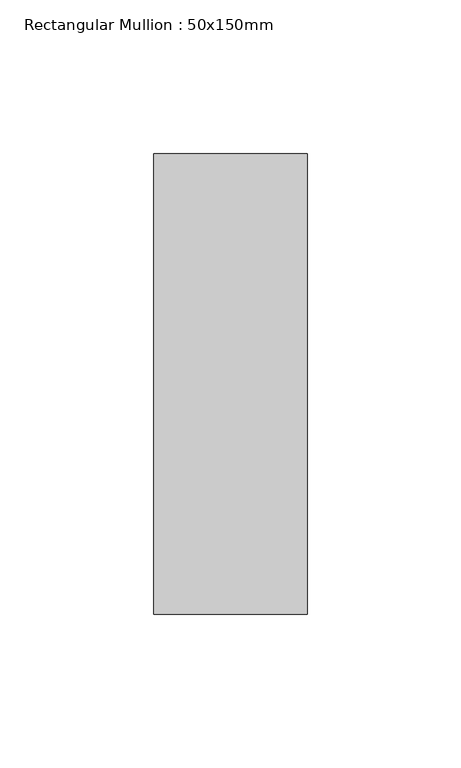
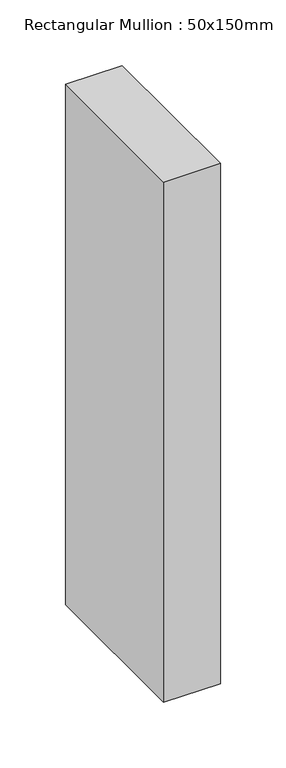
"""IFC4 building model written with IfcOpenShell, lengths in millimetres: member geometry, Rectangular Mullion : 50x150mm."""

from ifc_helpers import new_model, si_unit, frame, origin, place, context, project, spatial, polyline, outline, extrude, source, transform, mapped, element, save


def rectangular_mullion_50x150mm_bddf6eb5(model_context):
    return source(origin(), model_context, "Body", "SweptSolid", [
        extrude(outline(polyline([(0.0, 75.0), (0.0, -75.0), (-50.0, -75.0), (-50.0, 75.0), (0.0, 75.0)])), frame((0.0, 0.0, -484.2), z_axis=(0.0, 0.0, 1.0), x_axis=(1.0, 0.0, 0.0)), (0.0, 0.0, 1.0), 484.2),
    ])


if __name__ == "__main__":
    model = new_model("IFC4")
    model_context = context("Model", 3, world=origin())
    ifc_project = project(units=[si_unit("LENGTHUNIT", "METRE", prefix="MILLI")], contexts=[model_context])
    site = spatial("IfcSite", under=ifc_project)
    building = spatial("IfcBuilding", under=site)
    placement = place(None, origin())
    rectangular_mullion_50x150mm_shape = rectangular_mullion_50x150mm_bddf6eb5(model_context)
    element("IfcMember", 1, ObjectType="Rectangular Mullion : 50x150mm", at=placement, inside=building, context=model_context, shape_type="MappedRepresentation", body=[
        mapped(rectangular_mullion_50x150mm_shape, transform((0.0, 0.0, 0.0), x_axis=(1.0, 0.0, 0.0), y_axis=(0.0, 1.0, 0.0), z_axis=(0.0, 0.0, 1.0))),
    ])
    save(model, "model.ifc")

# Revit data of these elements
# Type "Rectangular Mullion : 50x150mm"
#   Keynote = "H11"
#   built-in parameter 1007304 = 0.492126 (stored number, unit not read)
#   built-in parameter 1007301 = 0.082021 (stored number, unit not read)
#   built-in parameter 1007300 = 0.082021 (stored number, unit not read)
# Element 1 (IfcMember, "Rectangular Mullion : 50x150mm")
#   Materials on its faces: "Aluminium"
# Materials
#   "Aluminium": class "Metal", colour RGB 247 247 247, transparency 0, Description = "Aluminium 6061", Cost = 0
